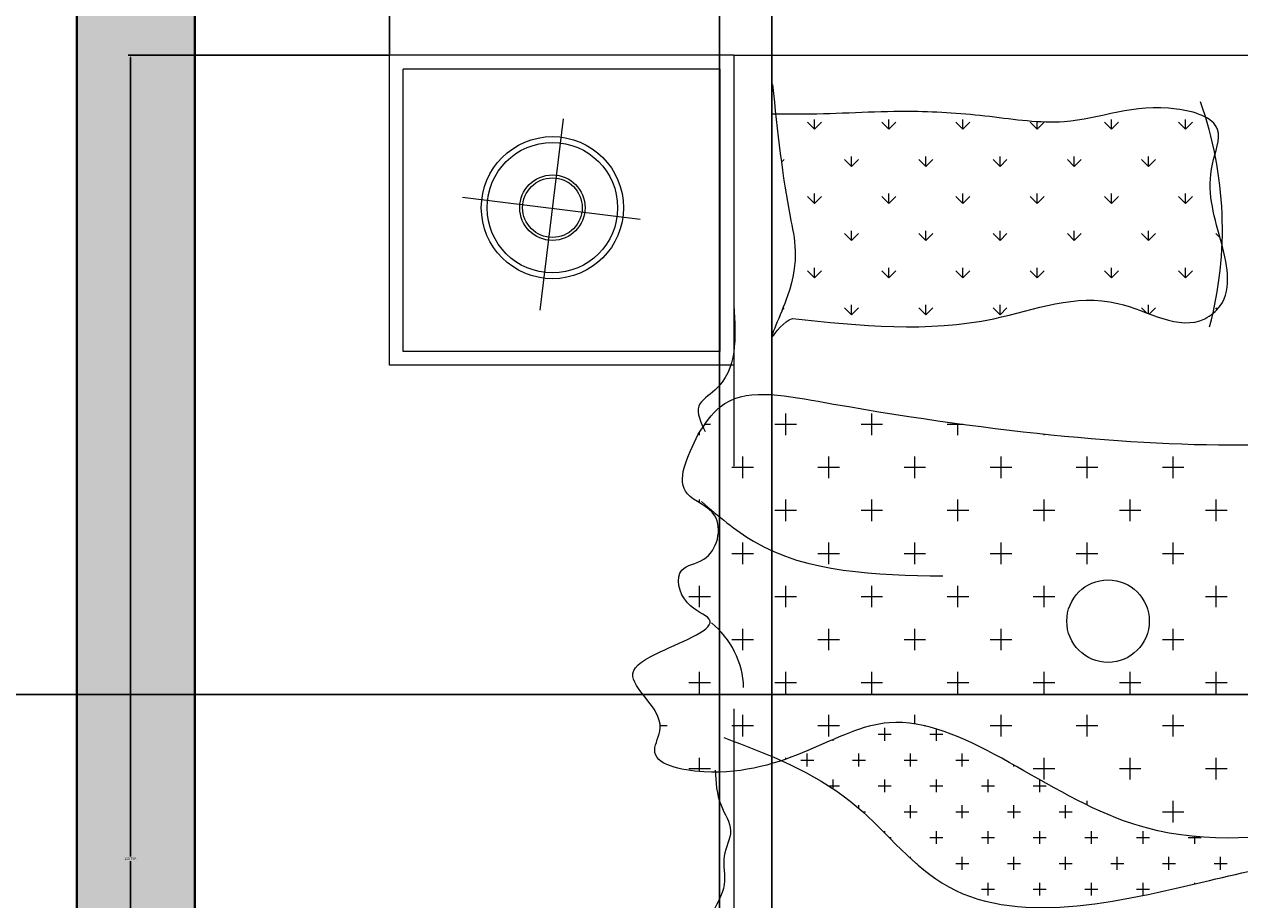
# Model space of a CAD drawing. Units: inches. Extents: x 2330 to 3943, y 1763 to 3461.
# Tile 5 of 40: x 2472 to 2564, y 2316 to 2383. Entities that reach past the tile are written whole.
import ezdxf

# ---------------------------------------------------------------- set-up
doc = ezdxf.new("R2010")
doc.units = ezdxf.units.IN
for name, color, linetype, lineweight in [('A-ANNO-DIMS', 2, 'Continuous', 18), ('A-FURN', 8, 'Continuous', 13), ('A-WALL', 7, 'Continuous', 40), ('A-WALL-PATT', 252, 'Continuous', 13)]:
    doc.layers.add(name, color=color, linetype=linetype, lineweight=lineweight)
doc.styles.get("Standard").update_dxf_attribs({"font": 'arial.ttf'})
doc.dimstyles.get("Standard").update_dxf_attribs({"dimtxt": 0.18, "dimasz": 0.18, "dimexe": 0.18, "dimexo": 0.0625, "dimgap": 0.09, "dimtad": 0, "dimtih": 1, "dimtoh": 1, "dimdec": 4, "dimzin": 0, "dimdsep": 46, "dimtxsty": 'Standard', "dimcen": 0.09, "dimadec": 0, "dimazin": 0, "dimtfac": 1, "dimtdec": 4, "dimtofl": 0, "dimtmove": 0, "dimatfit": 3, "dimfxl": 1, "dimtolj": 1, "dimtzin": 0, "dimarcsym": 0})

# ---------------------------------------------------------------- blocks, each defined once
blk = doc.blocks.new('A$C200C7901')
for p, q in [((0, 1.8834), (0, 2.3334)), ((0.5, 2.3334), (0, 2.3334)), ((0.5, 2.3334), (0.5, 1.7369)), ((0.5, 2.3334), (0.5, 1.7369)), ((0.5, 2.3334), (2, 2.3334)), ((0.9943, 2.1721), (0.9842, 2.1822)), ((0.9943, 2.1721), (0.9842, 2.1822)), ((0.9943, 2.0643), (0.9842, 2.0744)), ((0.9943, 2.0643), (0.9842, 2.0744)), ((1.206, 2.0681), (1.1997, 2.0744)), ((1.206, 2.0681), (1.1997, 2.0744)), ((0.5701, 1.9635), (0.5733, 1.9666)), ((0.5701, 1.9635), (0.5733, 1.9666)), ((1.2019, 1.9645), (1.1997, 1.9666)), ((1.2019, 1.9645), (1.1997, 1.9666)), ((0.5, 1.8834), (0, 1.8834)), ((0.4504, 1.782), (0.4504, 1.7863)), ((0.4504, 1.782), (0.4504, 1.7863)), ((0.458, 1.7977), (0.466, 1.7977)), ((0.458, 1.7977), (0.466, 1.7977)), ((1.1379, 1.7195), (1.1379, 1.7508)), ((1.1222, 1.7352), (1.1535, 1.7352)), ((0.4504, 1.6834), (0.4504, 1.6883)), ((0.4504, 1.6834), (0.4504, 1.6883)), ((0.4656, 1.6727), (0.466, 1.6727)), ((0.4656, 1.6727), (0.466, 1.6727)), ((0.5597, 1.6727), (0.591, 1.6727)), ((0.5597, 1.6727), (0.591, 1.6727)), ((1.0129, 1.5945), (1.0129, 1.6258)), ((1.0129, 1.5945), (1.0129, 1.6258)), ((0.4504, 1.532), (0.4504, 1.5633)), ((1.0754, 1.5625), (1.0754, 1.5633)), ((1.0754, 1.5625), (1.0754, 1.5633)), ((0.4347, 1.5477), (0.466, 1.5477)), ((0.6847, 1.5477), (0.716, 1.5477)), ((0.4347, 1.4227), (0.466, 1.4227)), ((0.5, 1.3845), (0.5, 0.3086)), ((0.3931, 1.3602), (0.4035, 1.3602)), ((0.3931, 1.3602), (0.4035, 1.3602)), ((0.4972, 1.3602), (0.5285, 1.3602)), ((0.4972, 1.3602), (0.5285, 1.3602)), ((0.4504, 1.2936), (0.4504, 1.3133)), ((0.4504, 1.2936), (0.4504, 1.3133)), ((0.4347, 1.2977), (0.466, 1.2977)), ((0.4347, 1.2977), (0.466, 1.2977))]:
    blk.add_line(p, q)
at = {"linetype": 'ByBlock'}
for p, q in [((0.02, 1.9034), (0.02, 2.3134)), ((0.48, 2.3134), (0.02, 2.3134)), ((0.48, 1.9034), (0.48, 2.3134)), ((0.2524, 2.2412), (0.2186, 1.9635)), ((0.6171, 2.2259), (0.607, 2.236)), ((0.6171, 2.2259), (0.607, 2.236)), ((0.6171, 2.2259), (0.6171, 2.2402)), ((0.6171, 2.2259), (0.6171, 2.2402)), ((0.6171, 2.2259), (0.6272, 2.236)), ((0.6171, 2.2259), (0.6272, 2.236)), ((0.7249, 2.2259), (0.7148, 2.236)), ((0.7249, 2.2259), (0.7148, 2.236)), ((0.7249, 2.2259), (0.7249, 2.2402)), ((0.7249, 2.2259), (0.7249, 2.2402)), ((0.7249, 2.2259), (0.735, 2.236)), ((0.7249, 2.2259), (0.735, 2.236)), ((0.8326, 2.2259), (0.8225, 2.236)), ((0.8326, 2.2259), (0.8225, 2.236)), ((0.8326, 2.2259), (0.8326, 2.2402)), ((0.8326, 2.2259), (0.8326, 2.2402)), ((0.8326, 2.2259), (0.8427, 2.236)), ((0.8326, 2.2259), (0.8427, 2.236)), ((0.9404, 2.2259), (0.9303, 2.236)), ((0.9404, 2.2259), (0.9303, 2.236)), ((0.9404, 2.2259), (0.9404, 2.2369)), ((0.9404, 2.2259), (0.9404, 2.2369)), ((0.9404, 2.2259), (0.9505, 2.236)), ((0.9404, 2.2259), (0.9505, 2.236)), ((1.0482, 2.2259), (1.0381, 2.236)), ((1.0482, 2.2259), (1.0381, 2.236)), ((1.0482, 2.2259), (1.0482, 2.2402)), ((1.0482, 2.2259), (1.0482, 2.2402)), ((1.0482, 2.2259), (1.0583, 2.236)), ((1.0482, 2.2259), (1.0583, 2.236)), ((1.1559, 2.2259), (1.1458, 2.236)), ((1.1559, 2.2259), (1.1458, 2.236)), ((1.1559, 2.2259), (1.1559, 2.2402)), ((1.1559, 2.2259), (1.1559, 2.2402)), ((1.1559, 2.2259), (1.166, 2.236)), ((1.1559, 2.2259), (1.166, 2.236)), ((0.5692, 2.178), (0.5733, 2.1822)), ((0.5692, 2.178), (0.5733, 2.1822)), ((0.671, 2.1721), (0.6609, 2.1822)), ((0.671, 2.1721), (0.6609, 2.1822)), ((0.671, 2.172), (0.671, 2.1863)), ((0.671, 2.172), (0.671, 2.1863)), ((0.671, 2.1721), (0.6811, 2.1822)), ((0.671, 2.1721), (0.6811, 2.1822)), ((0.7787, 2.1721), (0.7686, 2.1822)), ((0.7787, 2.1721), (0.7686, 2.1822)), ((0.7787, 2.172), (0.7787, 2.1863)), ((0.7787, 2.172), (0.7787, 2.1863)), ((0.7787, 2.1721), (0.7889, 2.1822)), ((0.7787, 2.1721), (0.7889, 2.1822)), ((0.8865, 2.1721), (0.8764, 2.1822)), ((0.8865, 2.1721), (0.8764, 2.1822)), ((0.8865, 2.172), (0.8865, 2.1863)), ((0.8865, 2.172), (0.8865, 2.1863)), ((0.8865, 2.1721), (0.8966, 2.1822)), ((0.8865, 2.1721), (0.8966, 2.1822)), ((0.9943, 2.172), (0.9943, 2.1863)), ((0.9943, 2.172), (0.9943, 2.1863)), ((0.9943, 2.1721), (1.0044, 2.1822)), ((0.9943, 2.1721), (1.0044, 2.1822)), ((1.102, 2.1721), (1.0919, 2.1822)), ((1.102, 2.1721), (1.0919, 2.1822)), ((1.102, 2.172), (1.102, 2.1863)), ((1.102, 2.172), (1.102, 2.1863)), ((1.102, 2.1721), (1.1121, 2.1822)), ((1.102, 2.1721), (1.1121, 2.1822)), ((0.3641, 2.0951), (0.1061, 2.1268)), ((0.6171, 2.1182), (0.607, 2.1283)), ((0.6171, 2.1182), (0.607, 2.1283)), ((0.6171, 2.1182), (0.6171, 2.1325)), ((0.6171, 2.1182), (0.6171, 2.1325)), ((0.6171, 2.1182), (0.6272, 2.1283)), ((0.6171, 2.1182), (0.6272, 2.1283)), ((0.7249, 2.1182), (0.7148, 2.1283)), ((0.7249, 2.1182), (0.7148, 2.1283)), ((0.7249, 2.1182), (0.7249, 2.1325)), ((0.7249, 2.1182), (0.7249, 2.1325)), ((0.7249, 2.1182), (0.735, 2.1283)), ((0.7249, 2.1182), (0.735, 2.1283)), ((0.8326, 2.1182), (0.8225, 2.1283)), ((0.8326, 2.1182), (0.8225, 2.1283)), ((0.8326, 2.1182), (0.8326, 2.1325)), ((0.8326, 2.1182), (0.8326, 2.1325)), ((0.8326, 2.1182), (0.8427, 2.1283)), ((0.8326, 2.1182), (0.8427, 2.1283)), ((0.9404, 2.1182), (0.9303, 2.1283)), ((0.9404, 2.1182), (0.9303, 2.1283)), ((0.9404, 2.1182), (0.9404, 2.1325)), ((0.9404, 2.1182), (0.9404, 2.1325)), ((0.9404, 2.1182), (0.9505, 2.1283)), ((0.9404, 2.1182), (0.9505, 2.1283)), ((1.0482, 2.1182), (1.0381, 2.1283)), ((1.0482, 2.1182), (1.0381, 2.1283)), ((1.0482, 2.1182), (1.0482, 2.1325)), ((1.0482, 2.1182), (1.0482, 2.1325)), ((1.0482, 2.1182), (1.0583, 2.1283)), ((1.0482, 2.1182), (1.0583, 2.1283)), ((1.1559, 2.1182), (1.1458, 2.1283)), ((1.1559, 2.1182), (1.1458, 2.1283)), ((1.1559, 2.1182), (1.1559, 2.1325)), ((1.1559, 2.1182), (1.1559, 2.1325)), ((1.1559, 2.1182), (1.166, 2.1283)), ((1.1559, 2.1182), (1.166, 2.1283)), ((0.671, 2.0643), (0.6609, 2.0744)), ((0.671, 2.0643), (0.6609, 2.0744)), ((0.671, 2.0643), (0.671, 2.0786)), ((0.671, 2.0643), (0.671, 2.0786)), ((0.671, 2.0643), (0.6811, 2.0744)), ((0.671, 2.0643), (0.6811, 2.0744)), ((0.7787, 2.0643), (0.7686, 2.0744)), ((0.7787, 2.0643), (0.7686, 2.0744)), ((0.7787, 2.0643), (0.7787, 2.0786)), ((0.7787, 2.0643), (0.7787, 2.0786)), ((0.7787, 2.0643), (0.7889, 2.0744)), ((0.7787, 2.0643), (0.7889, 2.0744)), ((0.8865, 2.0643), (0.8764, 2.0744)), ((0.8865, 2.0643), (0.8764, 2.0744)), ((0.8865, 2.0643), (0.8865, 2.0786)), ((0.8865, 2.0643), (0.8865, 2.0786)), ((0.8865, 2.0643), (0.8966, 2.0744)), ((0.8865, 2.0643), (0.8966, 2.0744)), ((0.9943, 2.0643), (0.9943, 2.0786)), ((0.9943, 2.0643), (0.9943, 2.0786)), ((0.9943, 2.0643), (1.0044, 2.0744)), ((0.9943, 2.0643), (1.0044, 2.0744)), ((1.102, 2.0643), (1.0919, 2.0744)), ((1.102, 2.0643), (1.0919, 2.0744)), ((1.102, 2.0643), (1.102, 2.0786)), ((1.102, 2.0643), (1.102, 2.0786)), ((1.102, 2.0643), (1.1121, 2.0744)), ((1.102, 2.0643), (1.1121, 2.0744)), ((0.6171, 2.0104), (0.607, 2.0205)), ((0.6171, 2.0104), (0.607, 2.0205)), ((0.6171, 2.0104), (0.6171, 2.0247)), ((0.6171, 2.0104), (0.6171, 2.0247)), ((0.6171, 2.0104), (0.6272, 2.0205)), ((0.6171, 2.0104), (0.6272, 2.0205)), ((0.7249, 2.0104), (0.7148, 2.0205)), ((0.7249, 2.0104), (0.7148, 2.0205)), ((0.7249, 2.0104), (0.7249, 2.0247)), ((0.7249, 2.0104), (0.7249, 2.0247)), ((0.7249, 2.0104), (0.735, 2.0205)), ((0.7249, 2.0104), (0.735, 2.0205)), ((0.8326, 2.0104), (0.8225, 2.0205)), ((0.8326, 2.0104), (0.8225, 2.0205)), ((0.8326, 2.0104), (0.8326, 2.0247)), ((0.8326, 2.0104), (0.8326, 2.0247)), ((0.8326, 2.0104), (0.8427, 2.0205)), ((0.8326, 2.0104), (0.8427, 2.0205)), ((0.9404, 2.0104), (0.9303, 2.0205)), ((0.9404, 2.0104), (0.9303, 2.0205)), ((0.9404, 2.0104), (0.9404, 2.0247)), ((0.9404, 2.0104), (0.9404, 2.0247)), ((0.9404, 2.0104), (0.9505, 2.0205)), ((0.9404, 2.0104), (0.9505, 2.0205)), ((1.0482, 2.0104), (1.0381, 2.0205)), ((1.0482, 2.0104), (1.0381, 2.0205)), ((1.0482, 2.0104), (1.0482, 2.0247)), ((1.0482, 2.0104), (1.0482, 2.0247)), ((1.0482, 2.0104), (1.0583, 2.0205)), ((1.0482, 2.0104), (1.0583, 2.0205)), ((1.1559, 2.0104), (1.1458, 2.0205)), ((1.1559, 2.0104), (1.1458, 2.0205)), ((1.1559, 2.0104), (1.1559, 2.0247)), ((1.1559, 2.0104), (1.1559, 2.0247)), ((1.1559, 2.0104), (1.166, 2.0205)), ((1.1559, 2.0104), (1.166, 2.0205)), ((0.671, 1.9565), (0.6609, 1.9666)), ((0.671, 1.9565), (0.6609, 1.9666)), ((0.671, 1.9565), (0.671, 1.9708)), ((0.671, 1.9565), (0.671, 1.9708)), ((0.671, 1.9565), (0.6811, 1.9666)), ((0.671, 1.9565), (0.6811, 1.9666)), ((0.7787, 1.9565), (0.7686, 1.9666)), ((0.7787, 1.9565), (0.7686, 1.9666)), ((0.7787, 1.9565), (0.7787, 1.9708)), ((0.7787, 1.9565), (0.7787, 1.9708)), ((0.7787, 1.9565), (0.7889, 1.9666)), ((0.7787, 1.9565), (0.7889, 1.9666)), ((0.8865, 1.9565), (0.8764, 1.9666)), ((0.8865, 1.9565), (0.8764, 1.9666)), ((0.8865, 1.9565), (0.8865, 1.9708)), ((0.8865, 1.9565), (0.8865, 1.9708)), ((0.8865, 1.9565), (0.8966, 1.9666)), ((0.8865, 1.9565), (0.8966, 1.9666)), ((1.0993, 1.9593), (1.0919, 1.9666)), ((1.0993, 1.9593), (1.0919, 1.9666)), ((1.102, 1.9583), (1.102, 1.9708)), ((1.102, 1.9583), (1.102, 1.9708)), ((1.1033, 1.9578), (1.1121, 1.9666)), ((1.1033, 1.9578), (1.1121, 1.9666)), ((0.48, 1.9034), (0.02, 1.9034)), ((0.5754, 1.782), (0.5754, 1.8133)), ((0.5754, 1.782), (0.5754, 1.8133)), ((0.7004, 1.782), (0.7004, 1.8133)), ((0.7004, 1.782), (0.7004, 1.8133)), ((0.5597, 1.7977), (0.591, 1.7977)), ((0.5597, 1.7977), (0.591, 1.7977)), ((0.6847, 1.7977), (0.716, 1.7977)), ((0.6847, 1.7977), (0.716, 1.7977)), ((0.8097, 1.7977), (0.8331, 1.7977)), ((0.8097, 1.7977), (0.8331, 1.7977)), ((0.8254, 1.782), (0.8254, 1.7987)), ((0.8254, 1.782), (0.8254, 1.7987)), ((0.9504, 1.782), (0.9504, 1.7836)), ((0.9504, 1.782), (0.9504, 1.7836)), ((0.5129, 1.7195), (0.5129, 1.7508)), ((0.5129, 1.7195), (0.5129, 1.7508)), ((0.6379, 1.7195), (0.6379, 1.7508)), ((0.6379, 1.7195), (0.6379, 1.7508)), ((0.7629, 1.7195), (0.7629, 1.7508)), ((0.7629, 1.7195), (0.7629, 1.7508)), ((0.8879, 1.7195), (0.8879, 1.7508)), ((0.8879, 1.7195), (0.8879, 1.7508)), ((1.0129, 1.7195), (1.0129, 1.7508)), ((1.0129, 1.7195), (1.0129, 1.7508)), ((1.1379, 1.7195), (1.1379, 1.7508)), ((0.4972, 1.7352), (0.5285, 1.7352)), ((0.4972, 1.7352), (0.5285, 1.7352)), ((0.6222, 1.7352), (0.6535, 1.7352)), ((0.6222, 1.7352), (0.6535, 1.7352)), ((0.7472, 1.7352), (0.7785, 1.7352)), ((0.7472, 1.7352), (0.7785, 1.7352)), ((0.8722, 1.7352), (0.9035, 1.7352)), ((0.8722, 1.7352), (0.9035, 1.7352)), ((0.9972, 1.7352), (1.0285, 1.7352)), ((0.9972, 1.7352), (1.0285, 1.7352)), ((1.1222, 1.7352), (1.1535, 1.7352)), ((0.5754, 1.657), (0.5754, 1.6883)), ((0.5754, 1.657), (0.5754, 1.6883)), ((0.7004, 1.657), (0.7004, 1.6883)), ((0.7004, 1.657), (0.7004, 1.6883)), ((0.8254, 1.657), (0.8254, 1.6883)), ((0.8254, 1.657), (0.8254, 1.6883)), ((0.9504, 1.657), (0.9504, 1.6883)), ((0.9504, 1.657), (0.9504, 1.6883)), ((1.0754, 1.657), (1.0754, 1.6883)), ((1.0754, 1.657), (1.0754, 1.6883)), ((1.2004, 1.657), (1.2004, 1.6883)), ((1.2004, 1.657), (1.2004, 1.6883)), ((0.6847, 1.6727), (0.716, 1.6727)), ((0.6847, 1.6727), (0.716, 1.6727)), ((0.8097, 1.6727), (0.841, 1.6727)), ((0.8097, 1.6727), (0.841, 1.6727)), ((0.9347, 1.6727), (0.966, 1.6727)), ((0.9347, 1.6727), (0.966, 1.6727)), ((1.0597, 1.6727), (1.091, 1.6727)), ((1.0597, 1.6727), (1.091, 1.6727)), ((1.1847, 1.6727), (1.216, 1.6727)), ((1.1847, 1.6727), (1.216, 1.6727)), ((0.5129, 1.5945), (0.5129, 1.6258)), ((0.5129, 1.5945), (0.5129, 1.6258)), ((0.6379, 1.5945), (0.6379, 1.6258)), ((0.6379, 1.5945), (0.6379, 1.6258)), ((0.7629, 1.5945), (0.7629, 1.6258)), ((0.7629, 1.5945), (0.7629, 1.6258)), ((0.8879, 1.5945), (0.8879, 1.6258)), ((0.8879, 1.5945), (0.8879, 1.6258)), ((1.1379, 1.5945), (1.1379, 1.6258)), ((1.1379, 1.5945), (1.1379, 1.6258)), ((0.4972, 1.6102), (0.5285, 1.6102)), ((0.4972, 1.6102), (0.5285, 1.6102)), ((0.6222, 1.6102), (0.6535, 1.6102)), ((0.6222, 1.6102), (0.6535, 1.6102)), ((0.7472, 1.6102), (0.7785, 1.6102)), ((0.7472, 1.6102), (0.7785, 1.6102)), ((0.8722, 1.6102), (0.9035, 1.6102)), ((0.8722, 1.6102), (0.9035, 1.6102)), ((0.9972, 1.6102), (1.0285, 1.6102)), ((0.9972, 1.6102), (1.0285, 1.6102)), ((1.1222, 1.6102), (1.1535, 1.6102)), ((1.1222, 1.6102), (1.1535, 1.6102)), ((0.4504, 1.532), (0.4504, 1.5633)), ((0.5754, 1.532), (0.5754, 1.5633)), ((0.5754, 1.532), (0.5754, 1.5633)), ((0.7004, 1.532), (0.7004, 1.5633)), ((0.7004, 1.532), (0.7004, 1.5633)), ((0.8254, 1.532), (0.8254, 1.5633)), ((0.8254, 1.532), (0.8254, 1.5633)), ((0.9504, 1.532), (0.9504, 1.5633)), ((0.9504, 1.532), (0.9504, 1.5633)), ((1.2004, 1.532), (1.2004, 1.5633)), ((1.2004, 1.532), (1.2004, 1.5633)), ((0.4347, 1.5477), (0.466, 1.5477)), ((0.5597, 1.5477), (0.591, 1.5477)), ((0.5597, 1.5477), (0.591, 1.5477)), ((0.6847, 1.5477), (0.716, 1.5477)), ((0.8097, 1.5477), (0.841, 1.5477)), ((0.8097, 1.5477), (0.841, 1.5477)), ((0.9347, 1.5477), (0.966, 1.5477)), ((0.9347, 1.5477), (0.966, 1.5477)), ((1.1847, 1.5477), (1.216, 1.5477)), ((1.1847, 1.5477), (1.216, 1.5477)), ((0.5129, 1.4695), (0.5129, 1.5008)), ((0.5129, 1.4695), (0.5129, 1.5008)), ((0.6379, 1.4695), (0.6379, 1.5008)), ((0.6379, 1.4695), (0.6379, 1.5008)), ((0.7629, 1.4695), (0.7629, 1.5008)), ((0.7629, 1.4695), (0.7629, 1.5008)), ((0.8879, 1.4695), (0.8879, 1.5008)), ((0.8879, 1.4695), (0.8879, 1.5008)), ((1.1379, 1.4695), (1.1379, 1.5008)), ((1.1379, 1.4695), (1.1379, 1.5008)), ((0.4972, 1.4852), (0.5285, 1.4852)), ((0.4972, 1.4852), (0.5285, 1.4852)), ((0.6222, 1.4852), (0.6535, 1.4852)), ((0.6222, 1.4852), (0.6535, 1.4852)), ((0.7472, 1.4852), (0.7785, 1.4852)), ((0.7472, 1.4852), (0.7785, 1.4852)), ((0.8722, 1.4852), (0.9035, 1.4852)), ((0.8722, 1.4852), (0.9035, 1.4852)), ((1.1222, 1.4852), (1.1535, 1.4852)), ((1.1222, 1.4852), (1.1535, 1.4852)), ((0.4504, 1.407), (0.4504, 1.4383)), ((0.4504, 1.407), (0.4504, 1.4383)), ((0.5754, 1.407), (0.5754, 1.4383)), ((0.5754, 1.407), (0.5754, 1.4383)), ((0.7004, 1.407), (0.7004, 1.4383)), ((0.7004, 1.407), (0.7004, 1.4383)), ((0.8254, 1.407), (0.8254, 1.4383)), ((0.8254, 1.407), (0.8254, 1.4383)), ((0.9504, 1.407), (0.9504, 1.4383)), ((0.9504, 1.407), (0.9504, 1.4383)), ((1.0754, 1.407), (1.0754, 1.4383)), ((1.0754, 1.407), (1.0754, 1.4383)), ((1.2004, 1.407), (1.2004, 1.4383)), ((1.2004, 1.407), (1.2004, 1.4383)), ((0.4347, 1.4227), (0.466, 1.4227)), ((0.5597, 1.4227), (0.591, 1.4227)), ((0.5597, 1.4227), (0.591, 1.4227)), ((0.6847, 1.4227), (0.716, 1.4227)), ((0.6847, 1.4227), (0.716, 1.4227)), ((0.8097, 1.4227), (0.841, 1.4227)), ((0.8097, 1.4227), (0.841, 1.4227)), ((0.9347, 1.4227), (0.966, 1.4227)), ((0.9347, 1.4227), (0.966, 1.4227)), ((1.0597, 1.4227), (1.091, 1.4227)), ((1.0597, 1.4227), (1.091, 1.4227)), ((1.1847, 1.4227), (1.216, 1.4227)), ((1.1847, 1.4227), (1.216, 1.4227)), ((0.5129, 1.3445), (0.5129, 1.3758)), ((0.5129, 1.3445), (0.5129, 1.3758)), ((0.6222, 1.3602), (0.6535, 1.3602)), ((0.6222, 1.3602), (0.6535, 1.3602)), ((0.6379, 1.3445), (0.6379, 1.3758)), ((0.6379, 1.3445), (0.6379, 1.3758)), ((0.7629, 1.3627), (0.7629, 1.3758)), ((0.7629, 1.3627), (0.7629, 1.3758)), ((0.7762, 1.3602), (0.7785, 1.3602)), ((0.7762, 1.3602), (0.7785, 1.3602)), ((0.8722, 1.3602), (0.9035, 1.3602)), ((0.8722, 1.3602), (0.9035, 1.3602)), ((0.8879, 1.3445), (0.8879, 1.3758)), ((0.8879, 1.3445), (0.8879, 1.3758)), ((0.9972, 1.3602), (1.0285, 1.3602)), ((0.9972, 1.3602), (1.0285, 1.3602)), ((1.0129, 1.3445), (1.0129, 1.3758)), ((1.0129, 1.3445), (1.0129, 1.3758)), ((1.1222, 1.3602), (1.1535, 1.3602)), ((1.1222, 1.3602), (1.1535, 1.3602)), ((1.1379, 1.3445), (1.1379, 1.3758)), ((1.1379, 1.3445), (1.1379, 1.3758)), ((0.7097, 1.3477), (0.7285, 1.3477)), ((0.7097, 1.3477), (0.7285, 1.3477)), ((0.7191, 1.3383), (0.7191, 1.357)), ((0.7191, 1.3383), (0.7191, 1.357)), ((0.7847, 1.3477), (0.8035, 1.3477)), ((0.7847, 1.3477), (0.8035, 1.3477)), ((0.7941, 1.3383), (0.7941, 1.3554)), ((0.7941, 1.3383), (0.7941, 1.3554)), ((0.6441, 1.3383), (0.6441, 1.3399)), ((0.6441, 1.3383), (0.6441, 1.3399)), ((0.5754, 1.3115), (0.5754, 1.3133)), ((0.5754, 1.3115), (0.5754, 1.3133)), ((0.5972, 1.3102), (0.616, 1.3102)), ((0.5972, 1.3102), (0.616, 1.3102)), ((0.6066, 1.3008), (0.6066, 1.3195)), ((0.6066, 1.3008), (0.6066, 1.3195)), ((0.6722, 1.3102), (0.691, 1.3102)), ((0.6722, 1.3102), (0.691, 1.3102)), ((0.6816, 1.3008), (0.6816, 1.3195)), ((0.6816, 1.3008), (0.6816, 1.3195)), ((0.7472, 1.3102), (0.766, 1.3102)), ((0.7472, 1.3102), (0.766, 1.3102)), ((0.7566, 1.3008), (0.7566, 1.3195)), ((0.7566, 1.3008), (0.7566, 1.3195)), ((0.8222, 1.3102), (0.841, 1.3102)), ((0.8222, 1.3102), (0.841, 1.3102)), ((0.8316, 1.3008), (0.8316, 1.3195)), ((0.8316, 1.3008), (0.8316, 1.3195)), ((0.9504, 1.282), (0.9504, 1.3133)), ((0.9504, 1.282), (0.9504, 1.3133)), ((1.0754, 1.282), (1.0754, 1.3133)), ((1.0754, 1.282), (1.0754, 1.3133)), ((1.2004, 1.282), (1.2004, 1.3133)), ((1.2004, 1.282), (1.2004, 1.3133)), ((0.9066, 1.3008), (0.9066, 1.3028)), ((0.9066, 1.3008), (0.9066, 1.3028)), ((0.9347, 1.2977), (0.966, 1.2977)), ((0.9347, 1.2977), (0.966, 1.2977)), ((1.0597, 1.2977), (1.091, 1.2977)), ((1.0597, 1.2977), (1.091, 1.2977)), ((1.1847, 1.2977), (1.216, 1.2977)), ((1.1847, 1.2977), (1.216, 1.2977)), ((0.6379, 1.2727), (0.6535, 1.2727)), ((0.6379, 1.2727), (0.6535, 1.2727)), ((0.6441, 1.2686), (0.6441, 1.282)), ((0.6441, 1.2686), (0.6441, 1.282)), ((0.7097, 1.2727), (0.7285, 1.2727)), ((0.7097, 1.2727), (0.7285, 1.2727)), ((0.7191, 1.2633), (0.7191, 1.282)), ((0.7191, 1.2633), (0.7191, 1.282)), ((0.7847, 1.2727), (0.8035, 1.2727)), ((0.7847, 1.2727), (0.8035, 1.2727)), ((0.7941, 1.2633), (0.7941, 1.282)), ((0.7941, 1.2633), (0.7941, 1.282)), ((0.8597, 1.2727), (0.8785, 1.2727)), ((0.8597, 1.2727), (0.8785, 1.2727)), ((0.8691, 1.2633), (0.8691, 1.282)), ((0.8691, 1.2633), (0.8691, 1.282)), ((0.9347, 1.2727), (0.9535, 1.2727)), ((0.9347, 1.2727), (0.9535, 1.2727)), ((0.9441, 1.2633), (0.9441, 1.2816)), ((0.9441, 1.2633), (0.9441, 1.2816)), ((0.6816, 1.2398), (0.6816, 1.2445)), ((0.6816, 1.2398), (0.6816, 1.2445)), ((0.6868, 1.2352), (0.691, 1.2352)), ((0.6868, 1.2352), (0.691, 1.2352)), ((0.7472, 1.2352), (0.766, 1.2352)), ((0.7472, 1.2352), (0.766, 1.2352)), ((0.7566, 1.2258), (0.7566, 1.2445)), ((0.7566, 1.2258), (0.7566, 1.2445)), ((0.8222, 1.2352), (0.841, 1.2352)), ((0.8222, 1.2352), (0.841, 1.2352)), ((0.8316, 1.2258), (0.8316, 1.2445)), ((0.8316, 1.2258), (0.8316, 1.2445)), ((0.8972, 1.2352), (0.916, 1.2352)), ((0.8972, 1.2352), (0.916, 1.2352)), ((0.9066, 1.2258), (0.9066, 1.2445)), ((0.9066, 1.2258), (0.9066, 1.2445)), ((0.9722, 1.2352), (0.991, 1.2352)), ((0.9722, 1.2352), (0.991, 1.2352)), ((0.9816, 1.2258), (0.9816, 1.2445)), ((0.9816, 1.2258), (0.9816, 1.2445)), ((1.0129, 1.2448), (1.0129, 1.2508)), ((1.0129, 1.2448), (1.0129, 1.2508)), ((1.1222, 1.2352), (1.1535, 1.2352)), ((1.1222, 1.2352), (1.1535, 1.2352)), ((1.1379, 1.2195), (1.1379, 1.2508)), ((1.1379, 1.2195), (1.1379, 1.2508)), ((0.7191, 1.2041), (0.7191, 1.207)), ((0.7191, 1.2041), (0.7191, 1.207)), ((0.7941, 1.1883), (0.7941, 1.207)), ((0.7941, 1.1883), (0.7941, 1.207)), ((0.8691, 1.1883), (0.8691, 1.207)), ((0.8691, 1.1883), (0.8691, 1.207)), ((0.9441, 1.1883), (0.9441, 1.207)), ((0.9441, 1.1883), (0.9441, 1.207)), ((1.0191, 1.1883), (1.0191, 1.207)), ((1.0191, 1.1883), (1.0191, 1.207)), ((1.0941, 1.1883), (1.0941, 1.207)), ((1.0941, 1.1883), (1.0941, 1.207)), ((0.7255, 1.1977), (0.7285, 1.1977)), ((0.7255, 1.1977), (0.7285, 1.1977)), ((0.7847, 1.1977), (0.8035, 1.1977)), ((0.7847, 1.1977), (0.8035, 1.1977)), ((0.8597, 1.1977), (0.8785, 1.1977)), ((0.8597, 1.1977), (0.8785, 1.1977)), ((0.9347, 1.1977), (0.9535, 1.1977)), ((0.9347, 1.1977), (0.9535, 1.1977)), ((1.0097, 1.1977), (1.0285, 1.1977)), ((1.0097, 1.1977), (1.0285, 1.1977)), ((1.0847, 1.1977), (1.1035, 1.1977)), ((1.0847, 1.1977), (1.1035, 1.1977)), ((1.1597, 1.1977), (1.1785, 1.1977)), ((1.1597, 1.1977), (1.1785, 1.1977)), ((1.1691, 1.1883), (1.1691, 1.1991)), ((1.1691, 1.1883), (1.1691, 1.1991)), ((0.7566, 1.1674), (0.7566, 1.1695)), ((0.7566, 1.1674), (0.7566, 1.1695)), ((0.8316, 1.1508), (0.8316, 1.1695)), ((0.8316, 1.1508), (0.8316, 1.1695)), ((0.9066, 1.1508), (0.9066, 1.1695)), ((0.9066, 1.1508), (0.9066, 1.1695)), ((0.9816, 1.1508), (0.9816, 1.1695)), ((0.9816, 1.1508), (0.9816, 1.1695)), ((1.0566, 1.1508), (1.0566, 1.1695)), ((1.0566, 1.1508), (1.0566, 1.1695)), ((1.1316, 1.1508), (1.1316, 1.1695)), ((1.1316, 1.1508), (1.1316, 1.1695)), ((1.2066, 1.1508), (1.2066, 1.1695)), ((1.2066, 1.1508), (1.2066, 1.1695)), ((0.7646, 1.1602), (0.766, 1.1602)), ((0.7646, 1.1602), (0.766, 1.1602)), ((0.8222, 1.1602), (0.841, 1.1602)), ((0.8222, 1.1602), (0.841, 1.1602)), ((0.8972, 1.1602), (0.916, 1.1602)), ((0.8972, 1.1602), (0.916, 1.1602)), ((0.9722, 1.1602), (0.991, 1.1602)), ((0.9722, 1.1602), (0.991, 1.1602)), ((1.0472, 1.1602), (1.066, 1.1602)), ((1.0472, 1.1602), (1.066, 1.1602)), ((1.1222, 1.1602), (1.141, 1.1602)), ((1.1222, 1.1602), (1.141, 1.1602)), ((1.1972, 1.1602), (1.216, 1.1602)), ((1.1972, 1.1602), (1.216, 1.1602)), ((0.8691, 1.1133), (0.8691, 1.132)), ((0.8691, 1.1133), (0.8691, 1.132)), ((0.9441, 1.1133), (0.9441, 1.132)), ((0.9441, 1.1133), (0.9441, 1.132)), ((1.0191, 1.1133), (1.0191, 1.132)), ((1.0191, 1.1133), (1.0191, 1.132)), ((1.0941, 1.1136), (1.0941, 1.132)), ((1.0941, 1.1136), (1.0941, 1.132)), ((1.1691, 1.1303), (1.1691, 1.132)), ((1.1691, 1.1303), (1.1691, 1.132)), ((0.8597, 1.1227), (0.8785, 1.1227)), ((0.8597, 1.1227), (0.8785, 1.1227)), ((0.9347, 1.1227), (0.9535, 1.1227)), ((0.9347, 1.1227), (0.9535, 1.1227)), ((1.0097, 1.1227), (1.0285, 1.1227)), ((1.0097, 1.1227), (1.0285, 1.1227)), ((1.0847, 1.1227), (1.1035, 1.1227)), ((1.0847, 1.1227), (1.1035, 1.1227))]:
    blk.add_line(p, q, dxfattribs=at)
for radius in [0.1032, 0.0947, 0.0475, 0.0432]:
    blk.add_circle((0.2367, 2.1121), radius, dxfattribs=at)
blk.add_circle((1.0433, 1.5119), 0.0599)
for centre, radius, start, end in [((0.658, 2.0811), 0.5513, 345.0722, 19.5492), ((0.3888, 1.4113), 0.1256, 1.9962, 51.1646)]:
    blk.add_arc(centre, radius, start, end)
blk.add_arc((0.3888, 1.4113), 0.1256, 1.9962, 51.1646, dxfattribs=at)
for points, knots in [([(0.5562, 2.2908), (0.5634, 2.223), (0.5751, 2.1147), (0.6005, 2.0213), (0.5392, 1.8966), (0.5726, 1.9486), (0.5854, 1.951)], [0, 0, 0, 0, 193.119101, 308.278592, 371.468985, 410.593498, 410.593498, 410.593498, 410.593498]), ([(0.5854, 1.951), (0.6835, 1.9407), (0.8425, 1.9242), (1.0374, 2.0054), (1.1564, 1.9255), (1.2274, 1.9841), (1.2052, 2.0751), (1.1815, 2.152), (1.2176, 2.2368), (1.0992, 2.2731), (1.0008, 2.2255), (0.8698, 2.246), (0.7481, 2.2548), (0.6426, 2.2473), (0.5746, 2.2478), (0.5562, 2.2479)], [0, 0, 0, 0, 292.165466, 473.33038, 601.631673, 630.723769, 727.138505, 836.819956, 887.958136, 954.42438, 1118.989809, 1227.016542, 1338.750986, 1487.447361, 1542.751028, 1542.751028, 1542.751028, 1542.751028]), ([(0.4485, 1.7835), (0.4321, 1.7496), (0.4062, 1.6964), (0.49, 1.6713), (0.4719, 1.5969), (0.4123, 1.592), (0.4233, 1.5337), (0.4954, 1.5086), (0.4012, 1.4738), (0.3253, 1.4306), (0.4113, 1.3764), (0.3688, 1.3065), (0.5579, 1.2663), (0.741, 1.4533), (1.1127, 1.1109), (1.4811, 1.2478), (1.7885, 1.3492), (2.0357, 1.1637), (2.0748, 1.2974), (2.0876, 1.349), (2.0192, 1.3805), (2.0564, 1.4298), (2.0588, 1.4846), (1.9759, 1.5349), (2.1004, 1.5845), (2.0397, 1.6519), (1.971, 1.7053), (2.1104, 1.8981), (1.5946, 1.7967), (1.2448, 1.7472), (0.8129, 1.7935), (0.4953, 1.8548), (0.4582, 1.7983), (0.4485, 1.7835)], [0, 0, 0, 0, 88.420092, 139.08588, 204.302936, 239.695496, 287.801042, 327.365471, 412.960499, 463.626286, 552.059846, 584.668336, 662.614915, 940.993281, 1309.926334, 1844.022653, 1996.276242, 2316.43048, 2341.441004, 2404.707416, 2449.463774, 2514.680778, 2538.40571, 2613.031547, 2697.13096, 2760.903931, 2822.692699, 2945.47, 3215.060018, 3725.584917, 4361.974444, 4504.671998, 4555.32777, 4555.32777, 4555.32777, 4555.32777]), ([(0.4856, 1.3429), (0.5504, 1.3182), (0.6715, 1.2721), (0.8374, 1.0498), (1.1164, 1.1183), (1.3878, 1.1816), (1.5888, 1.1102), (1.8403, 1.1127), (1.9415, 1.2178), (2.0032, 1.2819)], [0, 0, 0, 0, 205.411753, 383.654933, 772.067458, 921.644661, 1226.793228, 1388.983508, 1642.292305, 1642.292305, 1642.292305, 1642.292305])]:
    blk.add_open_spline(points, degree=3, knots=knots)
for points, knots in [([(0.5, 1.9703), (0.5029, 1.9235), (0.5066, 1.8648), (0.4398, 1.8252), (0.452, 1.8005), (0.4585, 1.7872)], [0, 0, 0, 0, 126.315232, 158.854004, 196.789047, 196.789047, 196.789047, 196.789047]), ([(0.5, 1.9703), (0.5029, 1.9235), (0.5066, 1.8648), (0.4398, 1.8252), (0.452, 1.8005), (0.4585, 1.7872)], [0, 0, 0, 0, 126.315232, 158.854004, 196.789047, 196.789047, 196.789047, 196.789047]), ([(0.4532, 1.6853), (0.4776, 1.6644), (0.574, 1.582), (0.7055, 1.5794), (0.8037, 1.5774)], [0, 0, 0, 0, 94.920667, 374.457292, 374.457292, 374.457292, 374.457292]), ([(0.4532, 1.6853), (0.4776, 1.6644), (0.574, 1.582), (0.7055, 1.5794), (0.8037, 1.5774)], [0, 0, 0, 0, 94.920667, 374.457292, 374.457292, 374.457292, 374.457292]), ([(0.473, 1.2954), (0.4739, 1.2781), (0.4755, 1.2477), (0.5032, 1.2084), (0.4801, 1.1701), (0.4928, 1.1255), (0.4674, 1.0912), (0.4579, 1.0351), (0.501, 0.9724), (0.4311, 0.8832), (0.4902, 0.8637), (0.4843, 0.8288), (0.4774, 0.7906), (0.4625, 0.7457), (0.459, 0.6999), (0.4816, 0.6664), (0.4748, 0.625), (0.4791, 0.5889), (0.4533, 0.5528), (0.4738, 0.5004), (0.4658, 0.4502), (0.4696, 0.3946), (0.4189, 0.3935), (0.4493, 0.3684), (0.4694, 0.3857), (0.4922, 0.3576), (0.5297, 0.3262), (0.5917, 0.3353), (0.6454, 0.3754), (0.7083, 0.3741), (0.7643, 0.3328), (0.826, 0.346), (0.925, 0.3388), (1.0353, 0.3593), (1.1561, 0.3744), (1.2477, 0.3154), (1.3302, 0.3474), (1.4086, 0.3512), (1.5217, 0.3878), (1.6362, 0.3176), (1.7682, 0.3285), (1.8402, 0.3019), (1.9071, 0.3529), (1.9647, 0.3412), (2.0795, 0.2948), (2.0472, 0.3498), (2.0343, 0.3772), (2.0435, 0.43), (2.0109, 0.5782), (2.0746, 0.4643), (2.0805, 0.584), (2.0084, 0.5979), (2.0343, 0.6846), (2.0344, 0.746), (2.0293, 0.8096), (2.0489, 0.8545), (2.0652, 0.9218), (1.9842, 0.9297), (2.0007, 1.0162), (2.0367, 1.0585), (2.0367, 1.1102), (2.0457, 1.1647), (2.0226, 1.2084), (2.0234, 1.2306), (2.0236, 1.2352)], [0, 0, 0, 0, 51.660678, 90.967412, 128.902454, 170.303599, 219.852997, 247.834962, 336.321557, 429.35469, 458.821847, 477.222321, 524.135809, 581.038434, 617.839381, 657.146115, 693.947125, 740.178081, 760.753248, 820.731705, 885.133458, 928.777044, 953.563729, 976.574207, 995.553042, 1018.563482, 1064.584401, 1147.951297, 1174.787598, 1266.851571, 1308.018447, 1377.066427, 1441.511314, 1608.245014, 1714.11869, 1792.771707, 1913.247991, 1954.931389, 2029.864445, 2259.189419, 2305.221512, 2429.507982, 2456.344283, 2543.92595, 2627.925037, 2662.96218, 2687.736879, 2719.937755, 2839.540991, 2875.47895, 2953.681041, 2993.270313, 3066.872333, 3154.395764, 3200.397042, 3248.426375, 3312.828127, 3347.881398, 3444.484026, 3481.577522, 3518.665244, 3592.267265, 3644.719162, 3658.519501, 3658.519501, 3658.519501, 3658.519501])]:
    blk.add_open_spline(points, degree=3, knots=knots, dxfattribs=at)
blk = doc.blocks.new('*D39')
at = {"layer": 'A-ANNO-DIMS', "color": 0, "lineweight": -2, "transparency": 16777216}
for p, q in [((2499.499, 2380.496), (2499.499, 2400.343)), ((2499.679, 2400.163), (2563.823, 2400.163)), ((2630.845, 2400.163), (2566.701, 2400.163)), ((2631.025, 2380.496), (2631.025, 2400.343))]:
    blk.add_line(p, q, dxfattribs=at)
at = {"layer": 'A-ANNO-DIMS', "color": 0, "transparency": 16777216}
for points in [[(2499.679, 2400.193), (2499.679, 2400.133), (2499.499, 2400.163)], [(2630.845, 2400.193), (2630.845, 2400.133), (2631.025, 2400.163)]]:
    blk.add_solid(points, dxfattribs=at)
at = {"layer": 'Defpoints', "color": 0, "transparency": 16777216}
for p in [(2631.025, 2400.163), (2499.499, 2380.434), (2631.025, 2380.434)]:
    blk.add_point(p, dxfattribs=at)
at = {"layer": 'A-ANNO-DIMS', "color": 0, "transparency": 16777216, "insert": (2565.262, 2400.163), "char_height": 0.18, "attachment_point": 5}
blk.add_mtext('\\A1;DOUBLE BED 132 TYP.', dxfattribs=at)
blk = doc.blocks.new('*D40')
at = {"layer": 'A-ANNO-DIMS', "color": 0, "lineweight": -2, "transparency": 16777216}
for p, q in [((2499.436, 2380.434), (2479.59, 2380.434)), ((2479.77, 2380.254), (2479.77, 2319.343)), ((2479.77, 2258.069), (2479.77, 2318.979)), ((2499.436, 2257.889), (2479.59, 2257.889))]:
    blk.add_line(p, q, dxfattribs=at)
at = {"layer": 'A-ANNO-DIMS', "color": 0, "transparency": 16777216}
for points in [[(2479.74, 2380.254), (2479.8, 2380.254), (2479.77, 2380.434)], [(2479.74, 2258.069), (2479.8, 2258.069), (2479.77, 2257.889)]]:
    blk.add_solid(points, dxfattribs=at)
at = {"layer": 'Defpoints', "color": 0, "transparency": 16777216}
for p in [(2479.77, 2380.434), (2499.499, 2380.434), (2499.499, 2257.889)]:
    blk.add_point(p, dxfattribs=at)
at = {"layer": 'A-ANNO-DIMS', "color": 0, "transparency": 16777216, "insert": (2479.77, 2319.161), "char_height": 0.18, "attachment_point": 5}
blk.add_mtext('\\A1;123 TYP.', dxfattribs=at)
blk = doc.blocks.new('*D62')
at = {"layer": 'A-ANNO-DIMS', "color": 0, "lineweight": -2, "transparency": 16777216}
for p, q in [((2475.598, 3162.652), (2330.502, 3162.652)), ((2330.682, 3162.472), (2330.682, 2687.584)), ((2330.682, 2212.332), (2330.682, 2687.221)), ((2475.598, 2212.152), (2330.502, 2212.152))]:
    blk.add_line(p, q, dxfattribs=at)
at = {"layer": 'A-ANNO-DIMS', "color": 0, "transparency": 16777216}
for points in [[(2330.652, 3162.472), (2330.712, 3162.472), (2330.682, 3162.652)], [(2330.652, 2212.332), (2330.712, 2212.332), (2330.682, 2212.152)]]:
    blk.add_solid(points, dxfattribs=at)
at = {"layer": 'Defpoints', "color": 0, "transparency": 16777216}
for p in [(2330.682, 3162.652), (2475.661, 3162.652), (2475.661, 2212.152)]:
    blk.add_point(p, dxfattribs=at)
at = {"layer": 'A-ANNO-DIMS', "color": 0, "transparency": 16777216, "insert": (2330.682, 2687.402), "char_height": 0.18, "attachment_point": 5}
blk.add_mtext('\\A1;950.5', dxfattribs=at)
blk = doc.blocks.new('*D79')
at = {"layer": 'A-ANNO-DIMS', "color": 0, "lineweight": -2, "transparency": 16777216}
for p, q in [((2484.661, 2221.215), (2484.661, 3461.303)), ((2484.841, 3461.123), (2504.438, 3461.123)), ((2524.481, 3461.123), (2504.883, 3461.123)), ((2524.661, 2221.215), (2524.661, 3461.303))]:
    blk.add_line(p, q, dxfattribs=at)
at = {"layer": 'A-ANNO-DIMS', "color": 0, "transparency": 16777216}
for points in [[(2484.841, 3461.153), (2484.841, 3461.093), (2484.661, 3461.123)], [(2524.481, 3461.153), (2524.481, 3461.093), (2524.661, 3461.123)]]:
    blk.add_solid(points, dxfattribs=at)
at = {"layer": 'Defpoints', "color": 0, "transparency": 16777216}
for p in [(2524.661, 3461.123), (2484.661, 2221.152), (2524.661, 2221.152)]:
    blk.add_point(p, dxfattribs=at)
at = {"layer": 'A-ANNO-DIMS', "color": 0, "transparency": 16777216, "insert": (2504.661, 3461.123), "char_height": 0.18, "attachment_point": 5}
blk.add_mtext('\\A1;40', dxfattribs=at)
blk = doc.blocks.new('*D80')
at = {"layer": 'A-ANNO-DIMS', "color": 0, "lineweight": -2, "transparency": 16777216}
for p, q in [((3166.598, 2331.698), (2330.502, 2331.698)), ((2330.682, 2331.518), (2330.682, 2322.357)), ((2330.682, 2312.832), (2330.682, 2321.993)), ((3166.598, 2312.652), (2330.502, 2312.652))]:
    blk.add_line(p, q, dxfattribs=at)
at = {"layer": 'A-ANNO-DIMS', "color": 0, "transparency": 16777216}
for points in [[(2330.652, 2331.518), (2330.712, 2331.518), (2330.682, 2331.698)], [(2330.652, 2312.832), (2330.712, 2312.832), (2330.682, 2312.652)]]:
    blk.add_solid(points, dxfattribs=at)
at = {"layer": 'Defpoints', "color": 0, "transparency": 16777216}
for p in [(2330.682, 2331.698), (3166.661, 2331.698), (3166.661, 2312.652)]:
    blk.add_point(p, dxfattribs=at)
at = {"layer": 'A-ANNO-DIMS', "color": 0, "transparency": 16777216, "insert": (2330.682, 2322.175), "char_height": 0.18, "attachment_point": 5}
blk.add_mtext('\\A1;19.046', dxfattribs=at)
blk = doc.blocks.new('*D90')
at = {"layer": 'A-ANNO-DIMS', "color": 0, "lineweight": -2, "transparency": 16777216}
for p, q in [((2484.661, 3153.59), (2484.661, 1901.197)), ((2528.661, 3153.59), (2528.661, 1901.197)), ((2484.841, 1901.377), (2506.438, 1901.377)), ((2528.481, 1901.377), (2506.883, 1901.377))]:
    blk.add_line(p, q, dxfattribs=at)
at = {"layer": 'A-ANNO-DIMS', "color": 0, "transparency": 16777216}
for points in [[(2484.841, 1901.407), (2484.841, 1901.347), (2484.661, 1901.377)], [(2528.481, 1901.407), (2528.481, 1901.347), (2528.661, 1901.377)]]:
    blk.add_solid(points, dxfattribs=at)
at = {"layer": 'Defpoints', "color": 0, "transparency": 16777216}
for p in [(2484.661, 3153.652), (2528.661, 3153.652), (2528.661, 1901.377)]:
    blk.add_point(p, dxfattribs=at)
at = {"layer": 'A-ANNO-DIMS', "color": 0, "transparency": 16777216, "insert": (2506.661, 1901.377), "char_height": 0.18, "attachment_point": 5}
blk.add_mtext('\\A1;44', dxfattribs=at)

msp = doc.modelspace()

# ---------------------------------------------------------------- hatches: boundary and pattern name
at = {"layer": 'A-WALL-PATT'}
h = msp.add_hatch(color=256, dxfattribs=at)
h.dxf.hatch_style = 1
h.paths.add_polyline_path([(2484.6605, 2499.7574), (2475.6605, 2499.7574), (2475.6605, 2212.1524), (2524.6605, 2212.1524), (2524.6605, 2221.1524), (2484.6605, 2221.1524), (2484.6605, 2385.1524), (2624.6605, 2385.1524), (2624.6605, 2422.1524), (2619.6605, 2422.1524), (2619.6605, 2390.1524), (2484.6605, 2390.1524), (2484.6605, 2462.1524), (2553.7039, 2462.1524), (2553.7039, 2467.1524), (2484.6605, 2467.1524)])

# ---------------------------------------------------------------- linework, layer by layer
at = {"layer": 'A-WALL'}
for p, q in [((2475.6605, 3162.6524), (2475.6605, 2212.1524)), ((2484.6605, 2385.1524), (2484.6605, 2221.1524))]:
    msp.add_line(p, q, dxfattribs=at)

# ---------------------------------------------------------------- block references
at = {"layer": 'A-FURN', "xscale": 52.5181391560459, "yscale": 52.5181391560459, "zscale": 52.5181391560459}
msp.add_blockref('A$C200C7901', (2499.4987, 2257.8888), dxfattribs=at)

# ---------------------------------------------------------------- dimensions: what is measured, and where the dimension line sits
at = {"layer": 'A-ANNO-DIMS'}
for base, p1, p2, picture, middle in [((2524.6605, 3461.1231), (2484.6605, 2221.1524), (2524.6605, 2221.1524), '*D79', (2504.6605, 3461.1231)), ((2528.6605, 1901.3774), (2484.6605, 3153.6524), (2528.6605, 3153.6524), '*D90', (2506.6605, 1901.3774))]:
    dim = msp.add_linear_dim(base=base, p1=p1, p2=p2, dimstyle='Standard', override={"dimdec": 0, "dimlfac": 1, "dimrnd": 0, "dimzin": 0, "dimdsep": 46, "dimlunit": 2}, dxfattribs=at)
    dim.commit()
    dim.dimension.update_dxf_attribs({"geometry": picture, "text_midpoint": middle})
for base, p1, p2, override, picture, middle in [((2330.6824, 3162.6524), (2475.6605, 2212.1524), (2475.6605, 3162.6524), {"dimdec": 1, "dimlfac": 1, "dimrnd": 0, "dimzin": 0, "dimdsep": 46, "dimlunit": 2}, '*D62', (2330.6824, 2687.4024)), ((2330.6824, 2331.6982), (3166.6605, 2312.6524), (3166.6605, 2331.6982), {"dimdec": 3, "dimlfac": 1, "dimrnd": 0, "dimzin": 0, "dimdsep": 46, "dimlunit": 2}, '*D80', (2330.6824, 2322.1753))]:
    dim = msp.add_linear_dim(base=base, p1=p1, p2=p2, angle=90, dimstyle='Standard', override=override, dxfattribs=at)
    dim.commit()
    dim.dimension.update_dxf_attribs({"geometry": picture, "text_midpoint": middle})
dim = msp.add_linear_dim(base=(2631.0254, 2400.1629), p1=(2499.4986, 2380.4339), p2=(2631.0254, 2380.4339), text='DOUBLE BED <> TYP.', dimstyle='Standard', override={"dimdec": 0, "dimlfac": 1, "dimrnd": 0, "dimzin": 0, "dimdsep": 46, "dimlunit": 2}, dxfattribs=at)
dim.commit()
dim.dimension.update_dxf_attribs({"geometry": '*D39', "text_midpoint": (2565.262, 2400.1629)})
dim = msp.add_linear_dim(base=(2479.7696, 2380.4339), p1=(2499.4986, 2257.8888), p2=(2499.4986, 2380.4339), angle=90, text='<> TYP.', dimstyle='Standard', override={"dimdec": 0, "dimlfac": 1, "dimrnd": 0, "dimzin": 0, "dimdsep": 46, "dimlunit": 2}, dxfattribs=at)
dim.commit()
dim.dimension.update_dxf_attribs({"geometry": '*D40', "text_midpoint": (2479.7696, 2319.1613)})

doc.saveas('drawing.dxf')
